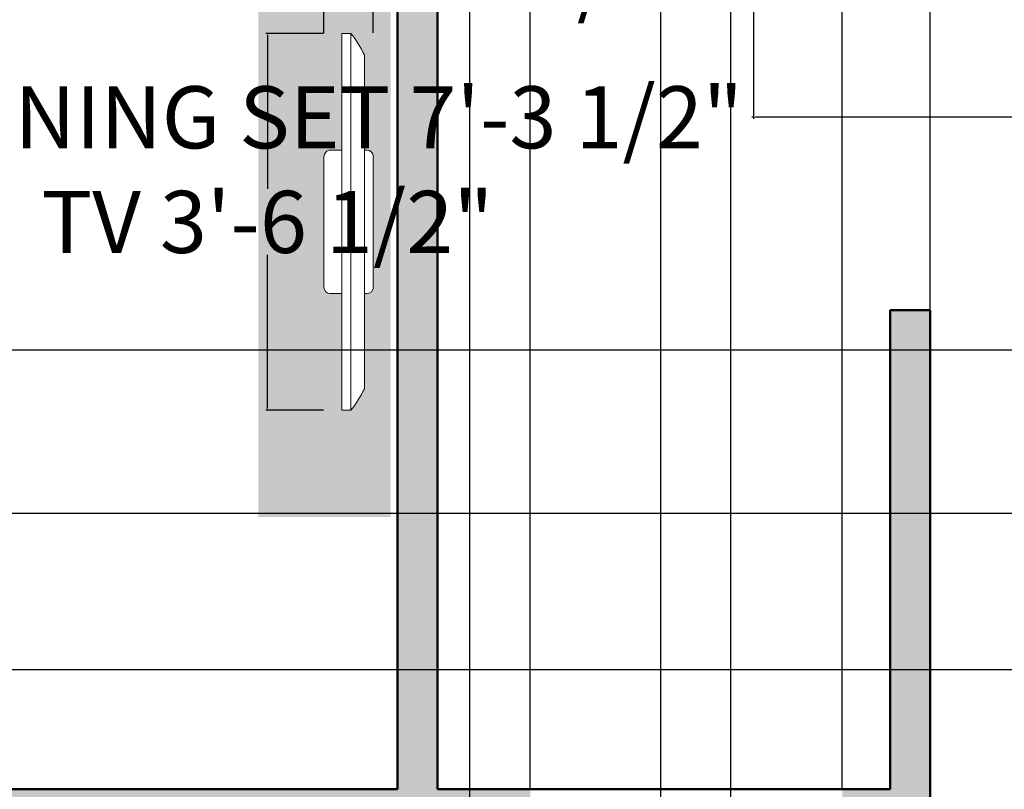
# Model space of a CAD drawing. Units: inches. Extents: x 2974 to 3443, y 2405 to 2963.
# Tile 3 of 13: x 3165 to 3276, y 2555 to 2642. Entities that reach past the tile are written whole.
import ezdxf

# ---------------------------------------------------------------- set-up
doc = ezdxf.new("R2010")
doc.units = ezdxf.units.IN
doc.header["$MEASUREMENT"] = 0
for name, color, linetype, lineweight in [('A-ANNO-DIMS', 2, 'Continuous', 18), ('A-EQPM', 32, 'Continuous', 20), ('A-WALL-PATT', 252, 'Continuous', 13), ('furniture', 32, 'Continuous', 18), ('walls', 250, 'Continuous', 50)]:
    doc.layers.add(name, color=color, linetype=linetype, lineweight=lineweight)
doc.layers.add('A-FURN-PATT', color=254, linetype='Continuous', lineweight=13, true_color=0xfeeab9)
doc.styles.get("Standard").update_dxf_attribs({"font": 'arial.ttf'})
doc.dimstyles.get("Standard").update_dxf_attribs({"dimtxt": 7, "dimasz": 0.18, "dimexe": 0.18, "dimexo": 0.0625, "dimgap": 0.09, "dimtad": 0, "dimtih": 1, "dimtoh": 1, "dimzin": 0, "dimdsep": 46, "dimlunit": 3, "dimtxsty": 'Standard', "dimcen": 0.09, "dimadec": 0, "dimazin": 0, "dimtfac": 1, "dimtofl": 0, "dimtmove": 0, "dimatfit": 3, "dimfxl": 1, "dimtolj": 1, "dimtzin": 0, "dimarcsym": 0})

# ---------------------------------------------------------------- blocks, each defined once
blk = doc.blocks.new('PLASMA-LARGE')
at = {"layer": 'furniture'}
for p, q in [((-7.26, 0), (7.26, 0)), ((-18.61, -1), (18.61, -1)), ((-8, -1), (-8, -0.74)), ((8, -1), (8, -0.74)), ((-21, -2.5), (21, -2.5)), ((-21, -2.5), (-21, -3.5)), ((21, -2.5), (21, -3.5)), ((-21, -3.5), (21, -3.5)), ((-8, -3.5), (-8, -4.76)), ((8, -3.5), (8, -4.76)), ((-7.26, -5.5), (7.26, -5.5))]:
    blk.add_line(p, q, dxfattribs=at)
for centre, radius, start, end in [((-7.26, -0.74), 0.744, 90, 180), ((7.26, -0.74), 0.744, 0, 90), ((-13.97, -11.05), 11.07, 114.7602, 129.4175), ((13.97, -11.05), 11.07, 50.5825, 65.2398), ((-7.26, -4.76), 0.744, 180, 270), ((7.26, -4.76), 0.744, 270, 0)]:
    blk.add_arc(centre, radius, start, end, dxfattribs=at)
blk = doc.blocks.new('*D45')
at = {"layer": 'A-ANNO-DIMS', "color": 0, "lineweight": -2, "transparency": 16777216}
for p, q in [((3198.99, 2640.39), (3192.5, 2640.39)), ((3192.68, 2640.21), (3192.68, 2622.87)), ((3192.68, 2598.1), (3192.68, 2615.44)), ((3198.99, 2597.92), (3192.5, 2597.92))]:
    blk.add_line(p, q, dxfattribs=at)
at = {"layer": 'A-ANNO-DIMS', "color": 0, "transparency": 16777216}
for points in [[(3192.65, 2640.21), (3192.71, 2640.21), (3192.68, 2640.39)], [(3192.65, 2598.1), (3192.71, 2598.1), (3192.68, 2597.92)]]:
    blk.add_solid(points, dxfattribs=at)
at = {"layer": 'Defpoints', "color": 0, "transparency": 16777216}
for p in [(3192.68, 2640.39), (3199.05, 2640.39), (3199.05, 2597.92)]:
    blk.add_point(p, dxfattribs=at)
at = {"layer": 'A-ANNO-DIMS', "color": 0, "transparency": 16777216, "insert": (3192.68, 2619.15), "char_height": 7, "attachment_point": 5}
blk.add_mtext('\\A1;TV 3\'-6 1/2"', dxfattribs=at)
blk = doc.blocks.new('*D46')
at = {"layer": 'A-ANNO-DIMS', "color": 0, "lineweight": -2, "transparency": 16777216}
for p, q in [((3199.05, 2640.45), (3199.05, 2646.94)), ((3199.23, 2646.76), (3204.43, 2646.76)), ((3204.61, 2640.45), (3204.61, 2646.94)), ((3204.61, 2646.76), (3204.79, 2646.76))]:
    blk.add_line(p, q, dxfattribs=at)
at = {"layer": 'A-ANNO-DIMS', "color": 0, "transparency": 16777216}
for points in [[(3199.23, 2646.79), (3199.23, 2646.73), (3199.05, 2646.76)], [(3204.43, 2646.79), (3204.43, 2646.73), (3204.61, 2646.76)]]:
    blk.add_solid(points, dxfattribs=at)
at = {"layer": 'Defpoints', "color": 0, "transparency": 16777216}
for p in [(3204.61, 2646.76), (3199.05, 2640.39), (3204.61, 2640.39)]:
    blk.add_point(p, dxfattribs=at)
at = {"layer": 'A-ANNO-DIMS', "color": 0, "transparency": 16777216, "insert": (3222.34, 2646.76), "char_height": 7, "attachment_point": 5}
blk.add_mtext('\\A1;0\'-5 1/2"', dxfattribs=at)
blk = doc.blocks.new('*D47')
at = {"layer": 'A-ANNO-DIMS', "color": 0, "lineweight": -2, "transparency": 16777216}
for p, q in [((3247.43, 2644.02), (3247.43, 2630.76)), ((3334.99, 2644.02), (3334.99, 2630.76)), ((3247.43, 2630.94), (3247.25, 2630.94)), ((3334.81, 2630.94), (3247.61, 2630.94))]:
    blk.add_line(p, q, dxfattribs=at)
at = {"layer": 'A-ANNO-DIMS', "color": 0, "transparency": 16777216}
for points in [[(3247.61, 2630.97), (3247.61, 2630.91), (3247.43, 2630.94)], [(3334.81, 2630.97), (3334.81, 2630.91), (3334.99, 2630.94)]]:
    blk.add_solid(points, dxfattribs=at)
at = {"layer": 'Defpoints', "color": 0, "transparency": 16777216}
for p in [(3247.43, 2644.08), (3334.99, 2644.08), (3247.43, 2630.94)]:
    blk.add_point(p, dxfattribs=at)
at = {"layer": 'A-ANNO-DIMS', "color": 0, "transparency": 16777216, "insert": (3200.53, 2630.94), "char_height": 7, "attachment_point": 5}
blk.add_mtext('\\A1;DINING SET 7\'-3 1/2"', dxfattribs=at)
blk = doc.blocks.new('*D61')
at = {"layer": 'A-ANNO-DIMS', "color": 0, "lineweight": -2, "transparency": 16777216}
for p, q in [((3222.29, 2555.25), (3222.29, 2952.68)), ((3257.43, 2555.25), (3257.43, 2952.68)), ((3222.47, 2952.5), (3227.69, 2952.5)), ((3257.25, 2952.5), (3252.03, 2952.5))]:
    blk.add_line(p, q, dxfattribs=at)
at = {"layer": 'A-ANNO-DIMS', "color": 0, "transparency": 16777216}
for points in [[(3222.47, 2952.53), (3222.47, 2952.47), (3222.29, 2952.5)], [(3257.25, 2952.53), (3257.25, 2952.47), (3257.43, 2952.5)]]:
    blk.add_solid(points, dxfattribs=at)
at = {"layer": 'Defpoints', "color": 0, "transparency": 16777216}
for p in [(3257.43, 2952.5), (3222.29, 2555.19), (3257.43, 2555.19)]:
    blk.add_point(p, dxfattribs=at)
at = {"layer": 'A-ANNO-DIMS', "color": 0, "transparency": 16777216, "insert": (3239.86, 2952.5), "char_height": 7, "attachment_point": 5}
blk.add_mtext('\\A1;2\'-11"', dxfattribs=at)
blk = doc.blocks.new('*D62')
at = {"layer": 'A-ANNO-DIMS', "color": 0, "lineweight": -2, "transparency": 16777216}
for p, q in [((3267.33, 2609.25), (3267.33, 2952.68)), ((3330, 2609.25), (3330, 2952.68)), ((3267.51, 2952.5), (3281.12, 2952.5)), ((3329.82, 2952.5), (3316.21, 2952.5))]:
    blk.add_line(p, q, dxfattribs=at)
at = {"layer": 'A-ANNO-DIMS', "color": 0, "transparency": 16777216}
for points in [[(3267.51, 2952.53), (3267.51, 2952.47), (3267.33, 2952.5)], [(3329.82, 2952.53), (3329.82, 2952.47), (3330, 2952.5)]]:
    blk.add_solid(points, dxfattribs=at)
at = {"layer": 'Defpoints', "color": 0, "transparency": 16777216}
for p in [(3330, 2952.5), (3267.33, 2609.19), (3330, 2609.19)]:
    blk.add_point(p, dxfattribs=at)
at = {"layer": 'A-ANNO-DIMS', "color": 0, "transparency": 16777216, "insert": (3298.66, 2952.5), "char_height": 7, "attachment_point": 5}
blk.add_mtext('\\A1;5\'-2 1/2"', dxfattribs=at)
blk = doc.blocks.new('*D63')
at = {"layer": 'A-ANNO-DIMS', "color": 0, "lineweight": -2, "transparency": 16777216}
for p, q in [((3244.83, 2751.13), (3244.83, 2414.92)), ((3284.83, 2751.13), (3284.83, 2414.92)), ((3245.01, 2415.1), (3255.43, 2415.1)), ((3284.65, 2415.1), (3274.22, 2415.1))]:
    blk.add_line(p, q, dxfattribs=at)
at = {"layer": 'A-ANNO-DIMS', "color": 0, "transparency": 16777216}
for points in [[(3245.01, 2415.13), (3245.01, 2415.07), (3244.83, 2415.1)], [(3284.65, 2415.13), (3284.65, 2415.07), (3284.83, 2415.1)]]:
    blk.add_solid(points, dxfattribs=at)
at = {"layer": 'Defpoints', "color": 0, "transparency": 16777216}
for p in [(3244.83, 2751.19), (3284.83, 2751.19), (3284.83, 2415.1)]:
    blk.add_point(p, dxfattribs=at)
at = {"layer": 'A-ANNO-DIMS', "color": 0, "transparency": 16777216, "insert": (3264.83, 2415.1), "char_height": 7, "attachment_point": 5}
blk.add_mtext('\\A1;3\'-4"', dxfattribs=at)
blk = doc.blocks.new('*D65')
at = {"layer": 'A-ANNO-DIMS', "color": 0, "lineweight": -2, "transparency": 16777216}
for p, q in [((3215.45, 2808.13), (3215.45, 2414.92)), ((3236.95, 2808.13), (3236.95, 2414.92)), ((3215.63, 2415.1), (3236.77, 2415.1)), ((3236.95, 2415.1), (3237.13, 2415.1))]:
    blk.add_line(p, q, dxfattribs=at)
at = {"layer": 'A-ANNO-DIMS', "color": 0, "transparency": 16777216}
for points in [[(3215.63, 2415.13), (3215.63, 2415.07), (3215.45, 2415.1)], [(3236.77, 2415.13), (3236.77, 2415.07), (3236.95, 2415.1)]]:
    blk.add_solid(points, dxfattribs=at)
at = {"layer": 'Defpoints', "color": 0, "transparency": 16777216}
for p in [(3215.45, 2808.19), (3236.95, 2808.19), (3236.95, 2415.1)]:
    blk.add_point(p, dxfattribs=at)
at = {"layer": 'A-ANNO-DIMS', "color": 0, "transparency": 16777216, "insert": (3254.35, 2415.1), "char_height": 7, "attachment_point": 5}
blk.add_mtext('\\A1;1\'-9 1/2"', dxfattribs=at)
blk = doc.blocks.new('*D73')
at = {"layer": 'A-ANNO-DIMS', "color": 0, "lineweight": -2, "transparency": 16777216}
for p, q in [((3329.94, 2604.69), (2992.84, 2604.69)), ((2993.02, 2604.51), (2993.02, 2599.19)), ((2993.02, 2586.45), (2993.02, 2591.77)), ((3330, 2586.27), (2992.84, 2586.27))]:
    blk.add_line(p, q, dxfattribs=at)
at = {"layer": 'A-ANNO-DIMS', "color": 0, "transparency": 16777216}
for points in [[(2992.99, 2604.51), (2993.05, 2604.51), (2993.02, 2604.69)], [(2992.99, 2586.45), (2993.05, 2586.45), (2993.02, 2586.27)]]:
    blk.add_solid(points, dxfattribs=at)
at = {"layer": 'Defpoints', "color": 0, "transparency": 16777216}
for p in [(2993.02, 2604.69), (3330, 2604.69), (3330.06, 2586.27)]:
    blk.add_point(p, dxfattribs=at)
at = {"layer": 'A-ANNO-DIMS', "color": 0, "transparency": 16777216, "insert": (2993.02, 2595.48), "char_height": 7, "attachment_point": 5}
blk.add_mtext('\\A1;1\'-6 1/2"', dxfattribs=at)
blk = doc.blocks.new('*D76')
at = {"layer": 'A-ANNO-DIMS', "color": 0, "lineweight": -2, "transparency": 16777216}
for p, q in [((3352.84, 2568.64), (2992.84, 2568.64)), ((2993.02, 2568.46), (2993.02, 2555.8)), ((2993.02, 2535.82), (2993.02, 2548.48)), ((3352.84, 2535.64), (2992.84, 2535.64))]:
    blk.add_line(p, q, dxfattribs=at)
at = {"layer": 'A-ANNO-DIMS', "color": 0, "transparency": 16777216}
for points in [[(2992.99, 2568.46), (2993.05, 2568.46), (2993.02, 2568.64)], [(2992.99, 2535.82), (2993.05, 2535.82), (2993.02, 2535.64)]]:
    blk.add_solid(points, dxfattribs=at)
at = {"layer": 'Defpoints', "color": 0, "transparency": 16777216}
for p in [(2993.02, 2568.64), (3352.9, 2568.64), (3352.9, 2535.64)]:
    blk.add_point(p, dxfattribs=at)
at = {"layer": 'A-ANNO-DIMS', "color": 0, "transparency": 16777216, "insert": (2993.02, 2552.14), "char_height": 7, "attachment_point": 5}
blk.add_mtext('\\A1;2\'-9"', dxfattribs=at)
blk = doc.blocks.new('*D78')
at = {"layer": 'A-ANNO-DIMS', "color": 0, "lineweight": -2, "transparency": 16777216}
for p, q in [((3267.33, 2480.25), (3267.33, 2952.68)), ((3310.86, 2481.93), (3310.86, 2952.68)), ((3267.51, 2952.5), (3271.55, 2952.5)), ((3310.68, 2952.5), (3306.64, 2952.5))]:
    blk.add_line(p, q, dxfattribs=at)
at = {"layer": 'A-ANNO-DIMS', "color": 0, "transparency": 16777216}
for points in [[(3267.51, 2952.53), (3267.51, 2952.47), (3267.33, 2952.5)], [(3310.68, 2952.53), (3310.68, 2952.47), (3310.86, 2952.5)]]:
    blk.add_solid(points, dxfattribs=at)
at = {"layer": 'Defpoints', "color": 0, "transparency": 16777216}
for p in [(3310.86, 2952.5), (3310.86, 2481.87), (3267.33, 2480.19)]:
    blk.add_point(p, dxfattribs=at)
at = {"layer": 'A-ANNO-DIMS', "color": 0, "transparency": 16777216, "insert": (3289.09, 2952.5), "char_height": 7, "attachment_point": 5}
blk.add_mtext('\\A1;3\'-7 1/2"', dxfattribs=at)

msp = doc.modelspace()

# ---------------------------------------------------------------- hatches: boundary and pattern name
at = {"layer": 'A-FURN-PATT'}
h = msp.add_hatch(color=256, dxfattribs=at)
h.dxf.hatch_style = 1
h.paths.add_polyline_path([(3191.663, 2650.336), (3206.56, 2650.336), (3206.56, 2585.893), (3191.663, 2585.893)])
h.paths.add_polyline_path([(3201.071, 2597.916), (3202.082, 2597.916, 0.0640419), (3203.599, 2600.336), (3203.599, 2611.063), (3203.857, 2611.063, 0.4142136), (3204.61, 2611.816), (3204.61, 2626.491, 0.4142136), (3203.857, 2627.244), (3203.599, 2627.244), (3203.599, 2637.972, 0.0640419), (3202.082, 2640.391), (3201.071, 2640.391), (3201.071, 2627.244), (3199.801, 2627.244, 0.4142136), (3199.048, 2626.491), (3199.048, 2611.816, 0.4142136), (3199.801, 2611.063), (3201.071, 2611.063)], flags=16)
at = {"layer": 'A-WALL-PATT'}
h = msp.add_hatch(color=256, dxfattribs=at)
h.dxf.hatch_style = 1
h.paths.add_polyline_path([(3222.294, 2555.188), (3211.826, 2555.188), (3211.826, 2657.938), (3207.326, 2657.938), (3207.326, 2555.188), (3051.326, 2555.188), (3051.326, 2583.943), (3042.326, 2583.943), (3042.326, 2471.188), (3165.027, 2471.188), (3165.027, 2480.188), (3051.326, 2480.188), (3051.326, 2550.688), (3222.294, 2550.688)])
h.paths.add_polyline_path([(3188.326, 2700.207), (3183.826, 2700.207), (3183.826, 2691.688), (3051.326, 2691.688), (3051.326, 2740.572), (3042.326, 2740.572), (3042.326, 2651.235), (3045.517, 2651.235), (3051.326, 2651.235), (3051.326, 2687.188), (3188.326, 2687.188)])
h.paths.add_polyline_path([(3051.326, 2894.188), (3074.298, 2894.188), (3074.298, 2903.188), (3042.326, 2903.188), (3042.326, 2807.864), (3045.517, 2807.864), (3051.326, 2807.864), (3051.326, 2835.688), (3103.457, 2835.688), (3103.457, 2839.066, -0.0124729), (3103.485, 2840.188), (3051.326, 2840.188)])
h.paths.add_polyline_path([(3201.987, 2903.188), (3100.263, 2903.188), (3100.263, 2894.188), (3131.326, 2894.188), (3131.326, 2835.688), (3135.826, 2835.688), (3135.826, 2894.188), (3183.826, 2894.188), (3183.826, 2840.188), (3159.826, 2840.188), (3159.826, 2835.688), (3183.826, 2835.688), (3183.826, 2740.207), (3188.326, 2740.207), (3188.326, 2803.688), (3215.422, 2803.688), (3215.422, 2807.066, -0.0124729), (3215.45, 2808.188), (3188.326, 2808.188), (3188.326, 2894.188), (3201.987, 2894.188)])
h.paths.add_polyline_path([(3283.564, 2903.188), (3227.952, 2903.188), (3227.952, 2894.188), (3240.326, 2894.188), (3240.326, 2755.688), (3188.326, 2755.688), (3188.326, 2751.188), (3244.826, 2751.188), (3244.826, 2757.188), (3244.826, 2797.188), (3244.826, 2894.188), (3283.564, 2894.188)])
h.paths.add_polyline_path([(3384.326, 2903.188), (3346.694, 2903.188), (3346.694, 2894.188), (3375.326, 2894.188), (3375.326, 2755.688), (3284.826, 2755.688), (3284.826, 2751.188), (3375.326, 2751.188), (3375.326, 2710.653), (3378.517, 2710.653), (3384.326, 2710.653)])
h.paths.add_polyline_path([(3384.326, 2643.361), (3375.326, 2643.361), (3375.326, 2609.188), (3330.003, 2609.188), (3330.003, 2604.688), (3375.326, 2604.688), (3375.326, 2480.188), (3356.49, 2480.188), (3356.49, 2471.188), (3384.326, 2471.188)])
h.paths.add_polyline_path([(3267.326, 2609.188), (3262.826, 2609.188), (3262.826, 2555.188), (3257.429, 2555.188), (3257.429, 2550.688), (3262.826, 2550.688), (3262.826, 2471.188), (3293.36, 2471.188), (3293.36, 2480.188), (3267.326, 2480.188)])
h.paths.add_polyline_path([(3275.186, 2471.188), (3268.471, 2471.188), (3268.471, 2455.229), (3268.471, 2452.413), (3275.186, 2452.413)])
h.paths.add_polyline_path([(3156.684, 2471.188), (3149.969, 2471.188), (3149.969, 2452.413), (3156.684, 2452.413)])

# ---------------------------------------------------------------- linework, layer by layer
at = {"layer": 'walls'}
for p, q in [((3207.326, 2555.188), (3207.326, 2657.938)), ((3211.826, 2555.188), (3211.826, 2657.938)), ((3262.826, 2609.188), (3267.326, 2609.188)), ((3262.826, 2609.188), (3262.826, 2555.188)), ((3267.326, 2609.188), (3267.326, 2480.188)), ((3051.326, 2555.188), (3207.326, 2555.188)), ((3211.826, 2555.188), (3262.826, 2555.188))]:
    msp.add_line(p, q, dxfattribs=at)

# ---------------------------------------------------------------- block references
at = {"layer": 'A-EQPM', "xscale": -1.011294184530666, "yscale": 1.011294184530666, "zscale": 1.011294184530666, "rotation": 270}
msp.add_blockref('PLASMA-LARGE', (3204.61, 2619.154), dxfattribs=at)

# ---------------------------------------------------------------- dimensions: what is measured, and where the dimension line sits
at = {"layer": 'A-ANNO-DIMS'}
for base, p1, p2, picture, middle in [((3330.003, 2952.498), (3267.326, 2609.188), (3330.003, 2609.188), '*D62', (3298.665, 2952.498)), ((3310.864, 2952.498), (3267.326, 2480.188), (3310.864, 2481.869), '*D78', (3289.095, 2952.498)), ((3257.429, 2952.498), (3222.294, 2555.188), (3257.429, 2555.188), '*D61', (3239.861, 2952.498)), ((3236.952, 2415.097), (3215.45, 2808.188), (3236.952, 2808.188), '*D65', (3254.352, 2415.097)), ((3284.826, 2415.097), (3244.826, 2751.188), (3284.826, 2751.188), '*D63', (3264.826, 2415.097)), ((3204.61, 2646.762), (3199.048, 2640.391), (3204.61, 2640.391), '*D46', (3222.339, 2646.762))]:
    dim = msp.add_linear_dim(base=base, p1=p1, p2=p2, dimstyle='Standard', override={"dimdec": 1, "dimlfac": 1, "dimrnd": 0, "dimzin": 1, "dimdsep": 46, "dimlunit": 4, "dimfrac": 2}, dxfattribs=at)
    dim.commit()
    dim.dimension.update_dxf_attribs({"geometry": picture, "text_midpoint": middle})
for base, p1, p2, angle, text, picture, middle in [((3247.425, 2630.944), (3334.991, 2644.079), (3247.425, 2644.079), 180, 'DINING SET <>', '*D47', (3200.531, 2630.944)), ((3192.677, 2640.391), (3199.048, 2597.916), (3199.048, 2640.391), 90, 'TV <>', '*D45', (3192.677, 2619.154))]:
    dim = msp.add_linear_dim(base=base, p1=p1, p2=p2, angle=angle, text=text, dimstyle='Standard', override={"dimdec": 1, "dimlfac": 1, "dimrnd": 0, "dimzin": 1, "dimdsep": 46, "dimlunit": 4, "dimfrac": 2}, dxfattribs=at)
    dim.commit()
    dim.dimension.update_dxf_attribs({"geometry": picture, "text_midpoint": middle})
for base, p1, p2, picture, middle in [((2993.016, 2604.688), (3330.059, 2586.273), (3330.003, 2604.688), '*D73', (2993.016, 2595.481)), ((2993.016, 2568.64), (3352.904, 2535.64), (3352.904, 2568.64), '*D76', (2993.016, 2552.14))]:
    dim = msp.add_linear_dim(base=base, p1=p1, p2=p2, angle=90, dimstyle='Standard', override={"dimdec": 1, "dimlfac": 1, "dimrnd": 0, "dimzin": 1, "dimdsep": 46, "dimlunit": 4, "dimfrac": 2}, dxfattribs=at)
    dim.commit()
    dim.dimension.update_dxf_attribs({"geometry": picture, "text_midpoint": middle})

doc.saveas('drawing.dxf')
